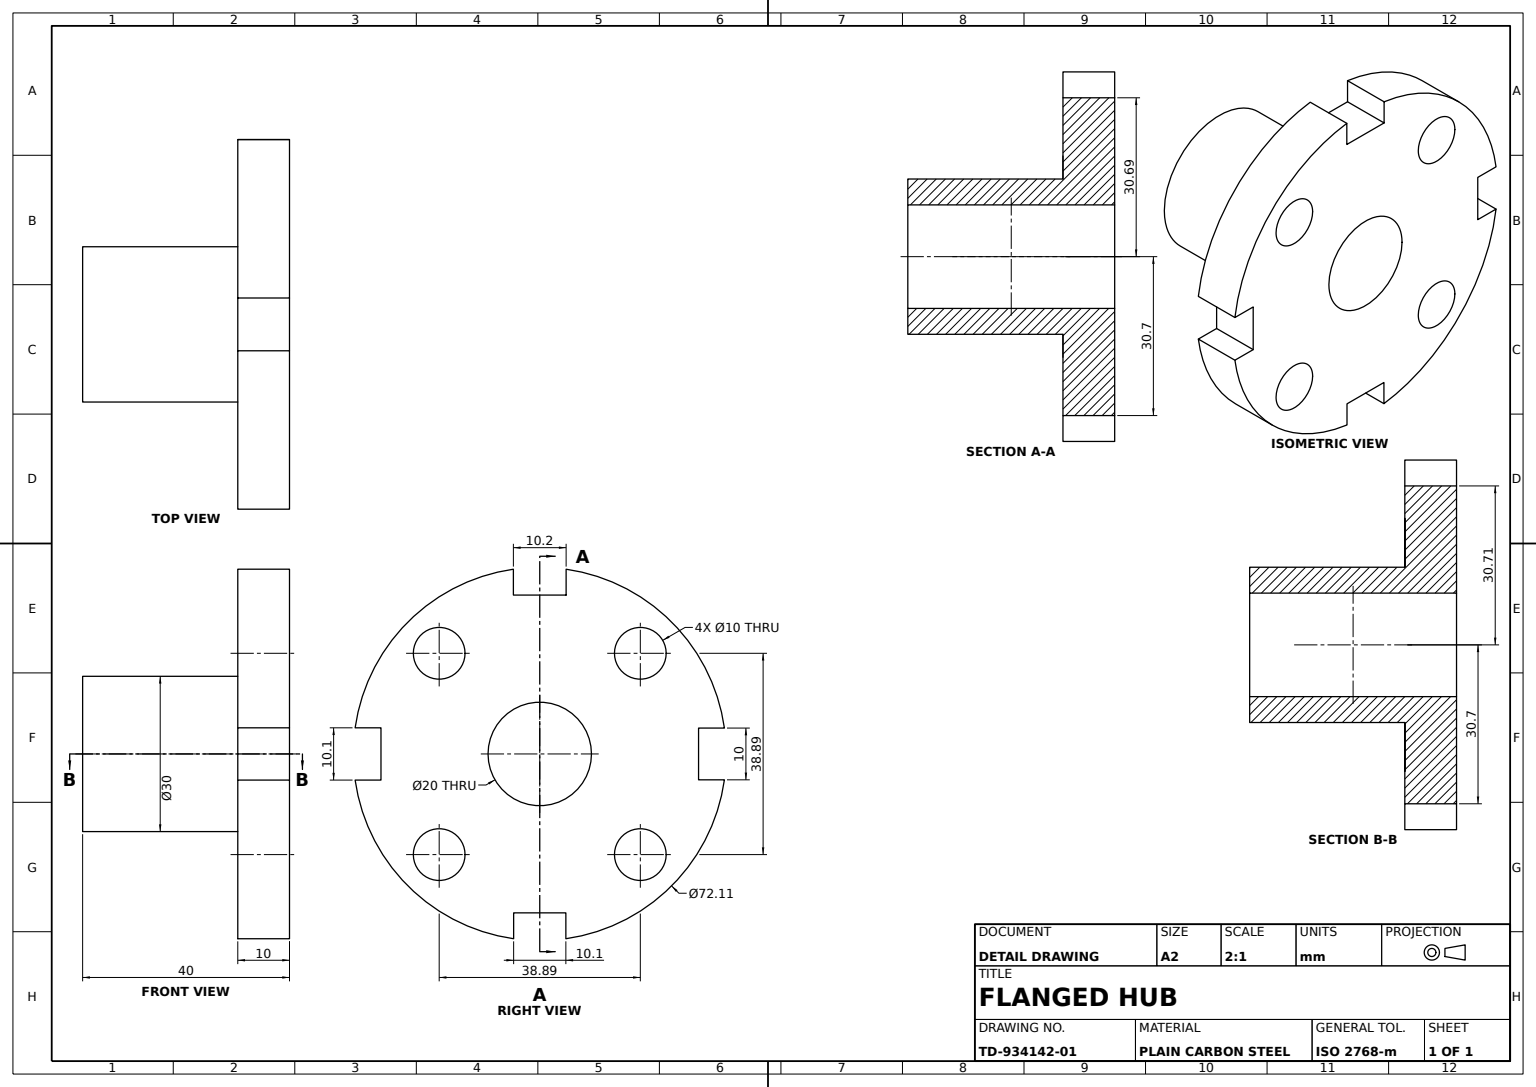
from build123d import *

# Parameters (mm, degrees)
FLANGE_PLATE_DEPTH         = 10
MOUNTING_HOLES_SKETCH_R    = 5
MOUNTING_HOLES_4X_10_DEPTH = 10
HUB_SKETCH_R               = 15
HUB_30_DEPTH               = 30
HUB_BORE_SKETCH_R          = 10
HUB_BORE_20_DEPTH          = 30
FLANGE_BORE_SKETCH_R       = 10
FLANGE_BORE_20_DEPTH       = 30


with BuildPart() as part:
    # Flange Profile Sketch → Flange Plate (new body)
    with BuildSketch(Plane.XY):
        with BuildLine():
            Line((0, 30.693136595), (5.099019514, 30.693136595))
            Line((5.099019514, 30.693136595), (5.099019514, 35.693136595))
            ThreePointArc((5.099019514, 35.693136595), (25.513031554, 25.477150958), (35.700277365, 5.048781643))
            Line((35.700277365, 5.048781643), (30.700277365, 5.048781643))
            Line((30.700277365, 5.048781643), (30.700277365, 0))
            Line((30.700277365, 0), (30.700277365, -5.048781643))
            Line((30.700277365, -5.048781643), (35.700277365, -5.048781643))
            ThreePointArc((35.700277365, -5.048781643), (25.495097568, -25.495097568), (5.048781643, -35.700277365))
            Line((5.048781643, -35.700277365), (5.048781643, -30.700277365))
            Line((5.048781643, -30.700277365), (0, -30.700277365))
            Line((0, -30.700277365), (-5.048781643, -30.700277365))
            Line((-5.048781643, -30.700277365), (-5.048781643, -35.700277365))
            ThreePointArc((-5.048781643, -35.700277365), (-25.512508471, -25.477674767), (-35.707142143, -5))
            Line((-35.707142143, -5), (-30.707142143, -5))
            Line((-30.707142143, -5), (-30.707142143, 0))
            Line((-30.707142143, 0), (-30.707142143, 5))
            Line((-30.707142143, 5), (-35.707142143, 5))
            ThreePointArc((-35.707142143, 5), (-25.530430192, 25.45971591), (-5.099019514, 35.693136595))
            Line((-5.099019514, 35.693136595), (-5.099019514, 30.693136595))
            Line((-5.099019514, 30.693136595), (0, 30.693136595))
        make_face()
    extrude(amount=FLANGE_PLATE_DEPTH)

    # Mounting Holes Sketch → Mounting Holes 4xØ10 (cut)
    with BuildSketch(Plane.XY.offset(10)):
        with Locations((19.445436483, 19.445436483)):
            Circle(MOUNTING_HOLES_SKETCH_R)
        with Locations((19.445436483, -19.445436483)):
            Circle(MOUNTING_HOLES_SKETCH_R)
        with Locations((-19.445436483, -19.445436483)):
            Circle(MOUNTING_HOLES_SKETCH_R)
        with Locations((-19.445436483, 19.445436483)):
            Circle(MOUNTING_HOLES_SKETCH_R)
    extrude(amount=-MOUNTING_HOLES_4X_10_DEPTH, mode=Mode.SUBTRACT)

    # Hub Sketch → Hub Ø30 (add)
    with BuildSketch(Plane.XY.offset(10)):
        Circle(HUB_SKETCH_R)
    extrude(amount=HUB_30_DEPTH)

    # Hub Bore Sketch → Hub Bore Ø20 (cut)
    with BuildSketch(Plane.XY.offset(40)):
        Circle(HUB_BORE_SKETCH_R)
    extrude(amount=-HUB_BORE_20_DEPTH, mode=Mode.SUBTRACT)

    # Flange Bore Sketch → Flange Bore Ø20 (cut)
    with BuildSketch(Plane.XY.offset(10)):
        Circle(FLANGE_BORE_SKETCH_R)
    extrude(amount=-FLANGE_BORE_20_DEPTH, mode=Mode.SUBTRACT)


solid = part.part
